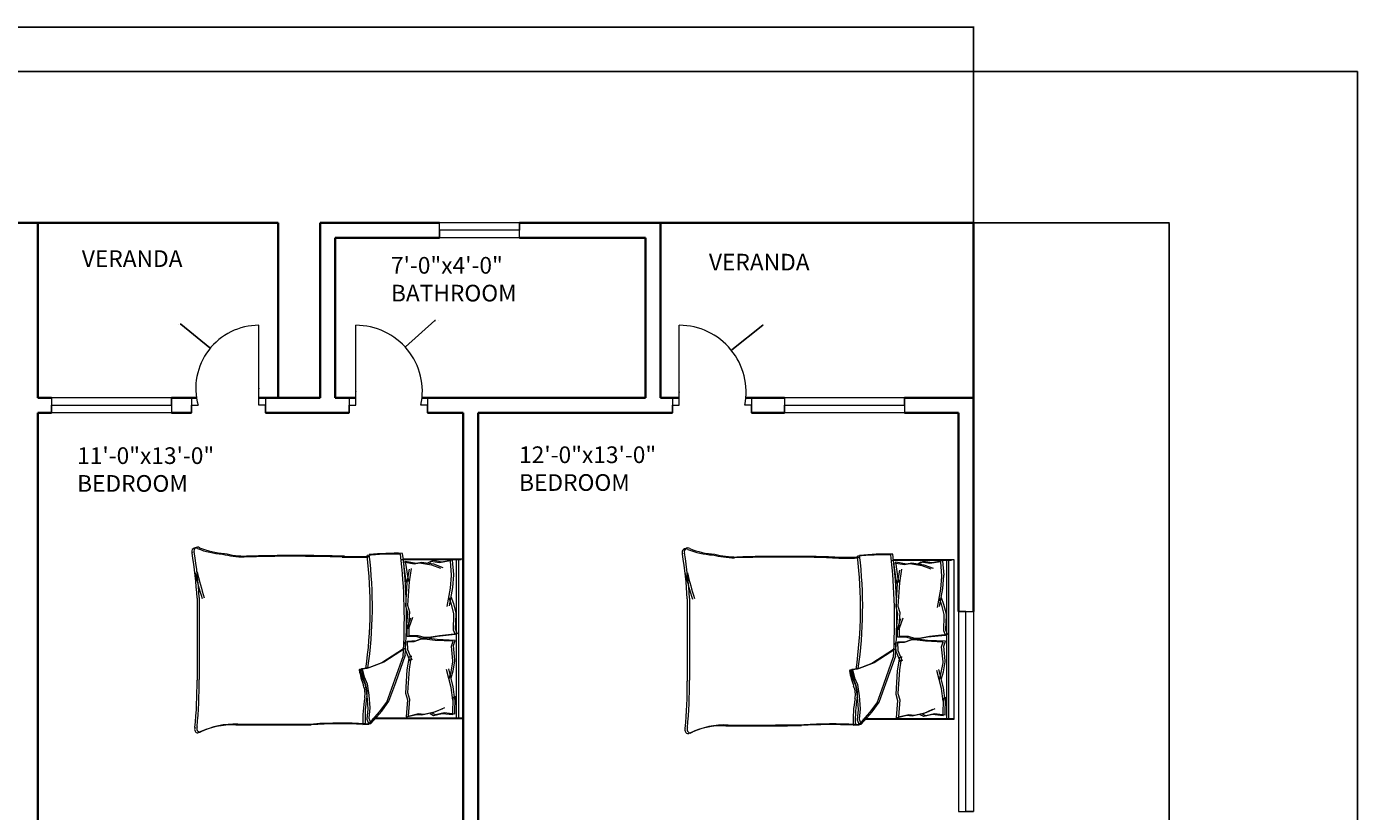
# Model space of a CAD drawing. Units: inches. Extents: x 2163 to 2982, y 1024 to 2288.
# Tile 22 of 22: x 2583 to 2982, y 2053 to 2288. Entities that reach past the tile are written whole.
import ezdxf

# ---------------------------------------------------------------- set-up
doc = ezdxf.new("R2010")
doc.units = ezdxf.units.IN
for name, color, linetype, lineweight in [('A-ANNO-DIMS', 2, 'Continuous', 18), ('A-ANNO-TTLB', 7, 'Continuous', 25), ('A-AREA-IDEN', 7, 'Continuous', 18), ('A-DOOR', 11, 'Continuous', 18), ('A-FURN', 8, 'Continuous', 13), ('A-GLAZ', 161, 'Continuous', 18), ('A-WALL', 7, 'Continuous', 35)]:
    doc.layers.add(name, color=color, linetype=linetype, lineweight=lineweight)
doc.styles.get("Standard").update_dxf_attribs({"font": 'arial.ttf'})
doc.dimstyles.get("Standard").update_dxf_attribs({"dimtxt": 0.18, "dimasz": 0.18, "dimexe": 0.18, "dimexo": 0.0625, "dimgap": 0.09, "dimtad": 0, "dimtih": 1, "dimtoh": 1, "dimdec": 4, "dimzin": 0, "dimdsep": 46, "dimtxsty": 'Standard', "dimcen": 0.09, "dimadec": 0, "dimazin": 0, "dimtfac": 1, "dimtdec": 4, "dimtofl": 0, "dimtmove": 0, "dimatfit": 3, "dimfxl": 1, "dimtolj": 1, "dimtzin": 0, "dimarcsym": 0})

# ---------------------------------------------------------------- blocks, each defined once
blk = doc.blocks.new('BED-DOUBLE')
for p, q in [((27.75, 52.87), (24.5, 49.16)), ((27.75, 52.87), (24.5, 49.16)), ((28.38, 53.1), (25.13, 49.39)), ((28.38, 53.1), (25.13, 49.39)), ((29.49, 52.95), (27.75, 52.87, 3.87)), ((29.49, 52.95), (27.75, 52.87, 3.87)), ((28.36, 51.33), (27.75, 52.87)), ((28.36, 51.33), (27.75, 52.87)), ((30.13, 53.18), (28.38, 53.1, 3.87)), ((29, 51.56), (28.38, 53.1)), ((30.13, 53.18), (28.38, 53.1, 3.87)), ((29, 51.56), (28.38, 53.1)), ((0, 51.49), (0.64, 51.49)), ((0, 3.47), (0, 51.49)), ((0, 51.27), (26.61, 51.27)), ((0, 51.27), (26.61, 51.27)), ((0.64, 51.49), (27.25, 51.49)), ((0.64, 51.49), (27.25, 51.49)), ((1.53, 3.48), (1.53, 51.27)), ((1.53, 3.47), (1.53, 51.27)), ((2.17, 3.7), (2.17, 51.49)), ((2.17, 3.7), (2.17, 51.49)), ((2.56, 50.11), (2.46, 44.71)), ((2.56, 50.11), (2.46, 44.71)), ((2.56, 50.11), (5.77, 49.73)), ((2.56, 50.11), (5.77, 49.73)), ((3.2, 50.34), (3.1, 44.94)), ((3.2, 50.34), (3.1, 44.94)), ((3.2, 50.34), (6.41, 49.96)), ((3.2, 50.34), (6.41, 49.96)), ((8.26, 49.31), (5.58, 48.13)), ((8.26, 49.31), (5.58, 48.13)), ((5.77, 49.73), (8.34, 50.33)), ((5.77, 49.73), (8.34, 50.33)), ((8.9, 49.54), (6.22, 48.36)), ((8.9, 49.54), (6.22, 48.36)), ((6.41, 49.96), (8.98, 50.56)), ((6.41, 49.96), (8.98, 50.56)), ((11.83, 50.11), (8.26, 49.31)), ((11.83, 50.11), (8.26, 49.31)), ((8.34, 50.33), (9.38, 49.81)), ((8.34, 50.33), (9.38, 49.81)), ((12.47, 50.34), (8.9, 49.54)), ((12.47, 50.34), (8.9, 49.54)), ((8.98, 50.56), (10.02, 50.04)), ((8.98, 50.56), (10.02, 50.04)), ((13.43, 49.92), (11.83, 50.11)), ((13.43, 49.92), (11.83, 50.11)), ((14.07, 50.15), (12.47, 50.34)), ((14.07, 50.15), (12.47, 50.34)), ((16.57, 50.7), (13.43, 49.92)), ((16.57, 50.7), (13.43, 49.92)), ((17.21, 50.93), (14.07, 50.15)), ((17.21, 50.93), (14.07, 50.15)), ((16.17, 45.57), (16.57, 50.7)), ((16.17, 45.57), (16.57, 50.7)), ((16.81, 45.79), (17.21, 50.93)), ((16.81, 45.79), (17.21, 50.93)), ((24.5, 49.16), (22.33, 46.22)), ((24.5, 49.16), (22.33, 46.22)), ((25.13, 49.39), (22.97, 46.45)), ((25.13, 49.39), (22.97, 46.45)), ((28.06, 48.23), (28.36, 51.33)), ((28.06, 48.23), (28.36, 51.33)), ((28.36, 44.36), (28.06, 48.23)), ((28.36, 44.36), (28.06, 48.23)), ((28.69, 48.46), (29, 51.56)), ((28.69, 48.46), (29, 51.56)), ((29, 44.59), (28.69, 48.46)), ((29, 44.59), (28.69, 48.46)), ((2.46, 44.71), (2.54, 45.71)), ((2.46, 44.71), (2.54, 45.71)), ((2.54, 45.71), (3.07, 41.91)), ((2.54, 45.71), (3.07, 41.91)), ((3.1, 44.94), (3.18, 45.94)), ((3.1, 44.94), (3.18, 45.94)), ((3.18, 45.94), (3.71, 42.14)), ((3.18, 45.94), (3.71, 42.14)), ((16.73, 43.61), (16.17, 45.57)), ((16.73, 43.61), (16.17, 45.57)), ((17.37, 43.83), (16.81, 45.79)), ((17.37, 43.83), (16.81, 45.79)), ((22.33, 46.22), (20.32, 40.64)), ((22.33, 46.22), (20.32, 40.64)), ((22.97, 46.45), (20.96, 40.87)), ((22.97, 46.45), (20.96, 40.87)), ((28.83, 40.95), (28.36, 44.36)), ((28.83, 40.95), (28.36, 44.36)), ((29.47, 41.18), (29, 44.59)), ((29.47, 41.18), (29, 44.59)), ((3.07, 41.91), (4.42, 36.49)), ((3.07, 41.91), (4.42, 36.49)), ((3.71, 42.14), (5.06, 36.72)), ((3.71, 42.14), (5.06, 36.72)), ((16.29, 36.6), (16.73, 43.61)), ((16.29, 36.6), (16.73, 43.61)), ((16.93, 36.82), (17.37, 43.83)), ((16.93, 36.82), (17.37, 43.83)), ((20.32, 40.64), (17.38, 32.31)), ((20.32, 40.64), (17.38, 32.31)), ((20.96, 40.87), (18.02, 32.53)), ((20.96, 40.87), (18.02, 32.53)), ((29.76, 38.94), (28.83, 40.95)), ((29.76, 38.94), (28.83, 40.95)), ((30.4, 39.17), (29.47, 41.18)), ((30.4, 39.17), (29.47, 41.18)), ((79.88, 15.29), (79.88, 39.91)), ((79.88, 15.29), (79.88, 39.91)), ((3.08, 37.14), (2.54, 34.2)), ((3.08, 37.13), (2.54, 34.2)), ((3.67, 39.2), (3.08, 37.14)), ((3.67, 39.2), (3.08, 37.13)), ((3.72, 37.36), (3.18, 34.43)), ((3.72, 37.36), (3.18, 34.43)), ((4.31, 39.43), (3.72, 37.36)), ((4.31, 39.43), (3.72, 37.36)), ((15.63, 32.56), (16.29, 36.6)), ((15.63, 32.56), (16.29, 36.6)), ((16.27, 32.79), (16.93, 36.82)), ((16.27, 32.79), (16.93, 36.82)), ((23.88, 34.45), (28.36, 36.15)), ((23.88, 34.45), (28.36, 36.15)), ((24.52, 34.68), (29, 36.38)), ((24.52, 34.68), (29, 36.38)), ((28.36, 36.15), (30.38, 36.46)), ((28.36, 36.15), (30.38, 36.46)), ((29, 36.38), (31.02, 36.69)), ((29, 36.38), (31.02, 36.69)), ((30.38, 36.46), (29.76, 38.94)), ((30.38, 36.46), (29.76, 38.94)), ((31.02, 36.69), (30.4, 39.17)), ((31.02, 36.69), (30.4, 39.17)), ((79.24, 15.06), (79.24, 39.68)), ((79.24, 15.06), (79.24, 39.68)), ((2.54, 34.2), (2.56, 33.88)), ((2.54, 34.2), (2.56, 33.88)), ((2.56, 33.88), (2.98, 29.46)), ((2.56, 33.88), (2.98, 29.46)), ((3.18, 34.43), (3.2, 34.11)), ((3.18, 34.43), (3.2, 34.11)), ((3.2, 34.11), (3.62, 29.68)), ((3.2, 34.11), (3.62, 29.68)), ((16.74, 30.75), (15.45, 33.82)), ((16.74, 30.75), (15.45, 33.82)), ((17.38, 30.98), (16.09, 34.05)), ((17.38, 30.98), (16.09, 34.05)), ((17.38, 30.26), (23.88, 34.45)), ((17.38, 30.26), (23.88, 34.45)), ((18.02, 30.49), (24.52, 34.68)), ((18.02, 30.49), (24.52, 34.68)), ((2.98, 29.46), (2.49, 27.98)), ((2.98, 29.46), (2.49, 27.98)), ((2.49, 27.98), (7.87, 27.73)), ((2.49, 27.98), (7.87, 27.73)), ((3.62, 29.68), (3.13, 28.21)), ((3.62, 29.68), (3.13, 28.2)), ((3.13, 28.21), (8.51, 27.96)), ((3.13, 28.2), (8.51, 27.96)), ((8.51, 27.96), (11.72, 27.58)), ((8.51, 27.96), (11.72, 27.58)), ((12.38, 27.44), (14.22, 28.13)), ((12.38, 27.44), (14.22, 28.13)), ((13.02, 27.66), (14.86, 28.36)), ((13.02, 27.66), (14.86, 28.36)), ((14.22, 28.13), (16.89, 28.3)), ((14.22, 28.13), (16.89, 28.3)), ((14.86, 28.36), (17.53, 28.53)), ((14.86, 28.36), (17.53, 28.53)), ((16.89, 28.3), (16.74, 30.75)), ((16.89, 28.3), (16.74, 30.75)), ((17.53, 28.53), (17.38, 30.98)), ((17.53, 28.53), (17.38, 30.98)), ((1.87, 25.98), (7.22, 26.56)), ((1.87, 25.98), (7.22, 26.56)), ((2.45, 24.54), (1.87, 25.98)), ((2.45, 24.54), (1.87, 25.98)), ((2.3, 20.09), (2.45, 24.54)), ((2.3, 20.09), (2.45, 24.54)), ((2.51, 26.21), (7.86, 26.79)), ((2.51, 26.21), (7.86, 26.79)), ((3.09, 24.77), (2.51, 26.21)), ((3.09, 24.77), (2.51, 26.21)), ((2.94, 20.32), (3.09, 24.77)), ((2.94, 20.32), (3.09, 24.77)), ((7.22, 26.56), (10.4, 27.14)), ((7.22, 26.56), (10.4, 27.14)), ((7.86, 26.79), (11.04, 27.37)), ((7.86, 26.79), (11.04, 27.37)), ((7.87, 27.73), (11.08, 27.35)), ((7.87, 27.73), (11.08, 27.35)), ((10.4, 27.14), (11.7, 27.14)), ((10.4, 27.14), (11.7, 27.14)), ((11.04, 27.37), (12.34, 27.37)), ((11.04, 27.37), (12.34, 27.37)), ((11.08, 27.35), (12.38, 27.44)), ((11.08, 27.35), (12.38, 27.44)), ((11.7, 27.14), (13.58, 26.56)), ((11.7, 27.14), (13.58, 26.56)), ((11.72, 27.58), (13.02, 27.66)), ((11.72, 27.58), (13.02, 27.66)), ((12.34, 27.37), (14.22, 26.79)), ((12.34, 27.37), (14.22, 26.79)), ((13.58, 26.56), (16.26, 26.56)), ((13.58, 26.56), (16.26, 26.56)), ((14.22, 26.79), (16.9, 26.79)), ((14.22, 26.79), (16.9, 26.79)), ((16.26, 24.1), (15.17, 20.96)), ((16.26, 24.1), (15.17, 20.96)), ((16.9, 24.33), (15.81, 21.19)), ((16.9, 24.33), (15.81, 21.19)), ((16.17, 19.38), (16.57, 24.52)), ((16.17, 19.38), (16.57, 24.52)), ((16.26, 26.56), (16.26, 24.1)), ((16.26, 26.56), (16.26, 24.1)), ((16.81, 19.61), (17.21, 24.74)), ((16.81, 19.61), (17.21, 24.74)), ((16.9, 26.79), (16.9, 24.33)), ((16.9, 26.79), (16.9, 24.33)), ((2.3, 19.77), (2.3, 20.09)), ((2.3, 19.77), (2.3, 20.09)), ((2.94, 20), (2.94, 20.32)), ((2.94, 20), (2.94, 20.32)), ((3.67, 17.11), (2.94, 20)), ((3.67, 17.11), (2.94, 20)), ((3.03, 16.88), (2.3, 19.77)), ((3.03, 16.88), (2.3, 19.77)), ((3.75, 14.85), (3.03, 16.88)), ((3.75, 14.85), (3.03, 16.88)), ((3.32, 12.11), (4.33, 17.6)), ((3.32, 12.11), (4.33, 17.6)), ((4.39, 15.08), (3.67, 17.11)), ((4.39, 15.08), (3.67, 17.11)), ((3.96, 12.34), (4.97, 17.83)), ((3.96, 12.34), (4.97, 17.83)), ((16.73, 17.42), (16.17, 19.38)), ((16.73, 17.42), (16.17, 19.38)), ((16.29, 10.41), (16.73, 17.42)), ((16.29, 10.41), (16.73, 17.42)), ((17.37, 17.65), (16.81, 19.61)), ((17.37, 17.65), (16.81, 19.61)), ((16.93, 10.64), (17.37, 17.65)), ((16.93, 10.64), (17.37, 17.65)), ((3.03, 8.28), (3.32, 12.11)), ((3.03, 8.28), (3.32, 12.11)), ((3.67, 8.51), (3.96, 12.34)), ((3.67, 8.51), (3.96, 12.34)), ((3.01, 8.18), (3.03, 8.28)), ((3.01, 8.18), (3.03, 8.28)), ((3.34, 3.9), (3.01, 8.18)), ((3.34, 3.9), (3.01, 8.18)), ((3.65, 8.41), (3.67, 8.51)), ((3.65, 8.41), (3.67, 8.51)), ((3.98, 4.13), (3.65, 8.41)), ((3.98, 4.13), (3.65, 8.41)), ((15.63, 6.38), (16.29, 10.41)), ((15.63, 6.38), (16.29, 10.41)), ((16.27, 6.61), (16.93, 10.64)), ((16.27, 6.61), (16.93, 10.64)), ((16.29, 10.41), (16.62, 9.28)), ((16.29, 10.41), (16.62, 9.28)), ((16.62, 9.28), (17.34, 4.18)), ((16.62, 9.28), (17.34, 4.18)), ((16.93, 10.64), (17.26, 9.51)), ((16.93, 10.64), (17.26, 9.51)), ((17.26, 9.51), (17.98, 4.41)), ((17.26, 9.51), (17.98, 4.41)), ((3.32, 3.89), (6.5, 4.47)), ((3.32, 3.89), (6.5, 4.47)), ((3.96, 4.12), (7.14, 4.7)), ((3.96, 4.12), (7.14, 4.7)), ((8.95, 5.05), (6.21, 6.06)), ((8.95, 5.05), (6.21, 6.06)), ((6.5, 4.47), (9.1, 4.04)), ((6.5, 4.47), (9.1, 4.04)), ((9.59, 5.28), (6.85, 6.29)), ((9.59, 5.28), (6.85, 6.29)), ((7.14, 4.7), (9.74, 4.27)), ((7.14, 4.7), (9.74, 4.27)), ((12.57, 4.47), (8.95, 5.05)), ((12.57, 4.47), (8.95, 5.05)), ((9.1, 4.04), (10.11, 4.62)), ((9.1, 4.04), (10.11, 4.62)), ((13.21, 4.7), (9.59, 5.28)), ((13.21, 4.7), (9.59, 5.28)), ((9.74, 4.27), (10.75, 4.85)), ((9.74, 4.27), (10.75, 4.85)), ((14.16, 4.76), (12.57, 4.47)), ((14.16, 4.76), (12.57, 4.47)), ((14.8, 4.99), (13.21, 4.7)), ((14.8, 4.99), (13.21, 4.7)), ((17.34, 4.18), (14.16, 4.76)), ((17.34, 4.18), (14.16, 4.76)), ((17.98, 4.41), (14.8, 4.99)), ((17.98, 4.41), (14.8, 4.99)), ((18.11, 3.48), (0, 3.48)), ((18.11, 3.47), (0, 3.47)), ((18.75, 3.7), (0.64, 3.7)), ((18.75, 3.7), (0.64, 3.7))]:
    blk.add_line(p, q)
for centre, radius, start, end in [((-6.66, 51.33), 36.18, 349.8763, 2.5657), ((-6.66, 51.33), 36.18, 349.8763, 2.5657), ((36.31, 182.27), 129.5, 266.9791, 273.8365), ((36.31, 182.27), 129.5, 266.9791, 273.8365), ((-6.02, 51.56), 36.18, 349.8763, 2.5657), ((-6.02, 51.56), 36.18, 349.8763, 2.5657), ((36.95, 182.49), 129.5, 266.9791, 273.8365), ((36.95, 182.49), 129.5, 266.9791, 273.8365), ((67.82, -4508.74), 4561.86, 90.00217, 90.28689), ((67.82, -4508.74), 4561.86, 90.00217, 90.28689), ((68.46, -4508.52), 4561.86, 90.00217, 90.28689), ((68.46, -4508.52), 4561.86, 90.00217, 90.28689), ((68.67, 76.16), 23.07, 267.4714, 296.4681), ((68.67, 76.16), 23.07, 267.4714, 296.4681), ((69.31, 76.39), 23.07, 267.4714, 296.4681), ((69.31, 76.39), 23.07, 267.4714, 296.4681), ((78.87, 54.41), 1.1, 332.6588, 86.02), ((78.87, 54.41), 1.1, 332.6588, 86.02), ((212.28, 41.15), 133.04, 174.4998, 180.6351), ((212.28, 41.15), 133.04, 174.4998, 180.6351), ((79.51, 54.64), 1.1, 332.6588, 86.02), ((79.51, 54.64), 1.1, 332.6588, 86.02), ((212.92, 41.38), 133.04, 174.4998, 180.6351), ((212.92, 41.38), 133.04, 174.4998, 180.6351), ((35.07, 43.74), 6.22, 168.6608, 203.7384), ((35.07, 43.74), 6.22, 168.6608, 203.7384), ((35.71, 43.97), 6.22, 168.6608, 203.7384), ((35.71, 43.97), 6.22, 168.6608, 203.7384), ((1.48, 31.15), 29.65, 10.6617, 19.8806), ((1.48, 31.15), 29.65, 10.6617, 19.8806), ((2.12, 31.38), 29.65, 10.6617, 19.8806), ((2.12, 31.38), 29.65, 10.6617, 19.8806), ((156.32, 17.76), 129.02, 171.7845, 186.9006), ((156.32, 17.76), 129.02, 171.7845, 186.9006), ((156.96, 17.98), 129.02, 171.7845, 186.9006), ((156.96, 17.98), 129.02, 171.7845, 186.9006), ((30.44, 36.64), 0.185, 250.2464, 1.1377), ((30.44, 36.64), 0.185, 250.2464, 1.1377), ((31.08, 36.86), 0.185, 250.2464, 1.1377), ((31.08, 36.86), 0.185, 250.2464, 1.1377), ((182.05, 21.36), 164.97, 176.0865, 186.7821), ((182.05, 21.36), 164.97, 176.0865, 186.7821), ((182.69, 21.59), 164.97, 176.0865, 186.7821), ((182.69, 21.59), 164.97, 176.0865, 186.7821), ((-23.71, -17.22), 106.46, 13.3832, 17.7053), ((-23.71, -17.22), 106.46, 13.3832, 17.7053), ((-23.07, -16.99), 106.46, 13.3832, 17.7053), ((-23.07, -16.99), 106.46, 13.3832, 17.7053), ((200.84, 21.43), 121.76, 182.9958, 189.4091), ((200.84, 21.43), 121.76, 182.9958, 189.4091), ((201.48, 21.66), 121.76, 182.9958, 189.4091), ((201.48, 21.65), 121.76, 182.9958, 189.4091), ((20.1, 85.16), 83.31, 268.7218, 275.604), ((20.1, 85.16), 83.31, 268.7218, 275.604), ((20.74, 85.39), 83.31, 268.7218, 275.604), ((20.74, 85.39), 83.31, 268.7218, 275.604), ((31.17, -167.31), 170.11, 88.4762, 91.0082), ((31.17, -167.31), 170.11, 88.4762, 91.0082), ((31.81, -167.08), 170.11, 88.4762, 91.0082), ((31.81, -167.08), 170.11, 88.4762, 91.0082), ((50.61, 484.82), 482.31, 268.2277, 271.7185), ((50.61, 484.82), 482.31, 268.2277, 271.7185), ((51.25, 485.05), 482.31, 268.2277, 271.7185), ((51.25, 485.05), 482.31, 268.2277, 271.7185), ((64.51, -26.9), 29.63, 76.0648, 88.9113), ((64.51, -26.9), 29.63, 76.0648, 88.9113), ((65.15, -26.67), 29.63, 76.0648, 88.9113), ((65.15, -26.67), 29.63, 76.0648, 88.9113), ((70.28, -21.66), 23.56, 67.9751, 86.652), ((70.28, -21.66), 23.56, 67.9751, 86.652), ((70.91, -21.43), 23.56, 67.9751, 86.652), ((70.91, -21.43), 23.56, 67.9751, 86.652), ((79.72, 1.09), 1.09, 236.1736, 23.4781), ((79.72, 1.09), 1.09, 236.1736, 23.4781), ((80.36, 1.32), 1.09, 236.1736, 23.4781), ((80.36, 1.32), 1.09, 236.1736, 23.4781)]:
    blk.add_arc(centre, radius, start, end)
blk = doc.blocks.new('WIN-24')
for p, q in [((0, 24), (4.5, 24)), ((0, 24), (0, 0)), ((4.5, 24), (2.25, 24)), ((2.25, 24), (2.25, 0)), ((4.5, 24), (4.5, 0)), ((2.25, 0), (0, 0)), ((0, 0), (4.5, 0))]:
    blk.add_line(p, q)
blk = doc.blocks.new('WIN-60')
for p, q in [((2.25, 60), (0, 60)), ((0, 60), (4.5, 60)), ((0, 60), (0, 0)), ((2.25, 0), (2.25, 60)), ((4.5, 60), (4.5, 0)), ((0, 0), (4.5, 0)), ((4.5, 0), (2.25, 0))]:
    blk.add_line(p, q)
blk = doc.blocks.new('WIN-36')
for p, q in [((2.25, 36), (0, 36)), ((0, 36), (4.5, 36)), ((0, 36), (0, 0)), ((2.25, 0), (2.25, 36)), ((4.5, 36), (4.5, 0)), ((0, 0), (4.5, 0)), ((4.5, 0), (2.25, 0))]:
    blk.add_line(p, q)
blk = doc.blocks.new('*D29')
at = {"layer": 'A-ANNO-DIMS', "color": 0, "lineweight": -2, "transparency": 16777216}
for p, q in [((2285.34, 1738.83), (2285.34, 2288.1)), ((2285.52, 2287.92), (2576.05, 2287.92)), ((2867.16, 2287.92), (2576.63, 2287.92)), ((2867.34, 2229.33), (2867.34, 2288.1))]:
    blk.add_line(p, q, dxfattribs=at)
at = {"layer": 'A-ANNO-DIMS', "color": 0, "transparency": 16777216}
for points in [[(2285.52, 2287.95), (2285.52, 2287.89), (2285.34, 2287.92)], [(2867.16, 2287.95), (2867.16, 2287.89), (2867.34, 2287.92)]]:
    blk.add_solid(points, dxfattribs=at)
at = {"layer": 'Defpoints', "color": 0, "transparency": 16777216}
for p in [(2867.34, 2287.92), (2867.34, 2229.27), (2285.34, 1738.77)]:
    blk.add_point(p, dxfattribs=at)
at = {"layer": 'A-ANNO-DIMS', "color": 0, "transparency": 16777216, "insert": (2576.34, 2287.92), "char_height": 0.18, "attachment_point": 5}
blk.add_mtext('\\A1;582', dxfattribs=at)
blk = doc.blocks.new('*D31')
at = {"layer": 'A-ANNO-DIMS', "color": 0, "lineweight": -2, "transparency": 16777216}
for p, q in [((2867.4, 2229.27), (2926.17, 2229.27)), ((2925.99, 2229.09), (2925.99, 1957.95)), ((2925.99, 1686.45), (2925.99, 1957.59)), ((2862.9, 1686.27), (2926.17, 1686.27))]:
    blk.add_line(p, q, dxfattribs=at)
at = {"layer": 'A-ANNO-DIMS', "color": 0, "transparency": 16777216}
for points in [[(2925.96, 2229.09), (2926.02, 2229.09), (2925.99, 2229.27)], [(2925.96, 1686.45), (2926.02, 1686.45), (2925.99, 1686.27)]]:
    blk.add_solid(points, dxfattribs=at)
at = {"layer": 'Defpoints', "color": 0, "transparency": 16777216}
for p in [(2867.34, 2229.27), (2925.99, 2229.27), (2862.84, 1686.27)]:
    blk.add_point(p, dxfattribs=at)
at = {"layer": 'A-ANNO-DIMS', "color": 0, "transparency": 16777216, "insert": (2925.99, 1957.77), "char_height": 0.18, "attachment_point": 5}
blk.add_mtext('\\A1;543', dxfattribs=at)
blk = doc.blocks.new('*D32')
at = {"layer": 'A-ANNO-DIMS', "color": 0, "lineweight": -2, "transparency": 16777216}
for p, q in [((2867.4, 2229.27), (2926.17, 2229.27)), ((2925.99, 2229.09), (2925.99, 1686.35)), ((2925.99, 1143.25), (2925.99, 1685.99)), ((2867.4, 1143.07), (2926.17, 1143.07))]:
    blk.add_line(p, q, dxfattribs=at)
at = {"layer": 'A-ANNO-DIMS', "color": 0, "transparency": 16777216}
for points in [[(2925.96, 2229.09), (2926.02, 2229.09), (2925.99, 2229.27)], [(2925.96, 1143.25), (2926.02, 1143.25), (2925.99, 1143.07)]]:
    blk.add_solid(points, dxfattribs=at)
at = {"layer": 'Defpoints', "color": 0, "transparency": 16777216}
for p in [(2867.34, 2229.27), (2925.99, 2229.27), (2867.34, 1143.07)]:
    blk.add_point(p, dxfattribs=at)
at = {"layer": 'A-ANNO-DIMS', "color": 0, "transparency": 16777216, "insert": (2925.99, 1686.17), "char_height": 0.18, "attachment_point": 5}
blk.add_mtext('\\A1;1086.2', dxfattribs=at)
blk = doc.blocks.new('*D60')
at = {"layer": 'A-ANNO-DIMS', "color": 0, "lineweight": -2, "transparency": 16777216}
for p, q in [((2629.52, 2198.81), (2629.7, 2198.81)), ((2629.7, 2198.81), (2638.35, 2191.71)), ((2653.04, 2179.57), (2653.22, 2179.57)), ((2653.13, 2179.48), (2653.13, 2179.66))]:
    blk.add_line(p, q, dxfattribs=at)
at = {"layer": 'A-ANNO-DIMS', "color": 0, "transparency": 16777216}
blk.add_solid([(2638.37, 2191.74), (2638.33, 2191.69), (2638.49, 2191.6)], dxfattribs=at)
at = {"layer": 'Defpoints', "color": 0, "transparency": 16777216}
for p in [(2638.49, 2191.6), (2653.13, 2179.57)]:
    blk.add_point(p, dxfattribs=at)
at = {"layer": 'A-ANNO-DIMS', "color": 0, "transparency": 16777216, "insert": (2628.98, 2198.81), "char_height": 0.18, "attachment_point": 5}
blk.add_mtext('\\A1;R18.944', dxfattribs=at)
blk = doc.blocks.new('*D61')
at = {"layer": 'A-ANNO-DIMS', "color": 0, "lineweight": -2, "transparency": 16777216}
for p, q in [((2705.83, 2199.99), (2697.09, 2192.09)), ((2706.01, 2199.99), (2705.83, 2199.99)), ((2682.1, 2178.59), (2682.28, 2178.59)), ((2682.19, 2178.5), (2682.19, 2178.68))]:
    blk.add_line(p, q, dxfattribs=at)
at = {"layer": 'A-ANNO-DIMS', "color": 0, "transparency": 16777216}
blk.add_solid([(2697.07, 2192.11), (2697.11, 2192.06), (2696.96, 2191.96)], dxfattribs=at)
at = {"layer": 'Defpoints', "color": 0, "transparency": 16777216}
for p in [(2696.96, 2191.96), (2682.19, 2178.59)]:
    blk.add_point(p, dxfattribs=at)
at = {"layer": 'A-ANNO-DIMS', "color": 0, "transparency": 16777216, "insert": (2706.49, 2199.99), "char_height": 0.18, "attachment_point": 5}
blk.add_mtext('\\A1;R19.93', dxfattribs=at)
blk = doc.blocks.new('*D62')
at = {"layer": 'A-ANNO-DIMS', "color": 0, "lineweight": -2, "transparency": 16777216}
for p, q in [((2804.16, 2198.55), (2794.92, 2191.13)), ((2804.34, 2198.55), (2804.16, 2198.55)), ((2779.06, 2178.47), (2779.24, 2178.47)), ((2779.15, 2178.38), (2779.15, 2178.56))]:
    blk.add_line(p, q, dxfattribs=at)
at = {"layer": 'A-ANNO-DIMS', "color": 0, "transparency": 16777216}
blk.add_solid([(2794.9, 2191.16), (2794.94, 2191.11), (2794.78, 2191.02)], dxfattribs=at)
at = {"layer": 'Defpoints', "color": 0, "transparency": 16777216}
for p in [(2794.78, 2191.02), (2779.15, 2178.47)]:
    blk.add_point(p, dxfattribs=at)
at = {"layer": 'A-ANNO-DIMS', "color": 0, "transparency": 16777216, "insert": (2804.82, 2198.55), "char_height": 0.18, "attachment_point": 5}
blk.add_mtext('\\A1;R20.05', dxfattribs=at)

msp = doc.modelspace()

# ---------------------------------------------------------------- linework, layer by layer
at = {"layer": 'A-ANNO-TTLB'}
msp.add_lwpolyline([(2162.6841, 2274.6054), (2982.469, 2274.6054), (2982.469, 1045.9691), (2162.6841, 1045.9691)], close=True, dxfattribs=at)
at = {"layer": 'A-DOOR'}
for p, q in [((2653.1269, 2174.5188), (2653.1269, 2198.5188)), ((2682.1865, 2174.5188), (2682.1865, 2198.5188)), ((2779.1453, 2174.5188), (2779.1453, 2198.5188)), ((2632.8695, 2176.7688), (2632.8695, 2172.2688)), ((2655.1269, 2176.7688), (2655.1269, 2172.2688)), ((2680.1865, 2176.7688), (2680.1865, 2172.2688)), ((2703.697, 2176.7688), (2703.697, 2172.2688)), ((2777.1453, 2176.7688), (2777.1453, 2172.2688)), ((2800.8036, 2176.7688), (2800.8036, 2172.2688)), ((2632.8695, 2172.2688), (2632.8695, 2174.5188)), ((2632.8695, 2174.5188), (2634.8695, 2174.5188)), ((2655.1269, 2174.5188), (2653.1269, 2174.5188)), ((2655.1269, 2172.2688), (2655.1269, 2174.5188)), ((2680.1865, 2172.2688), (2680.1865, 2174.5188)), ((2680.1865, 2174.5188), (2682.1865, 2174.5188)), ((2703.697, 2174.5188), (2701.697, 2174.5188)), ((2703.697, 2172.2688), (2703.697, 2174.5188)), ((2777.1453, 2172.2688), (2777.1453, 2174.5188)), ((2777.1453, 2174.5188), (2779.1453, 2174.5188)), ((2800.8036, 2174.5188), (2798.8036, 2174.5188)), ((2800.8036, 2172.2688), (2800.8036, 2174.5188))]:
    msp.add_line(p, q, dxfattribs=at)
for centre, radius, start, end in [((2653.1269, 2179.5744), 18.9444, 90, 195.477728), ((2682.1865, 2178.5885), 19.9304, 348.21777, 90), ((2779.1453, 2178.4679), 20.0509, 348.641269, 90)]:
    msp.add_arc(centre, radius, start, end, dxfattribs=at)
at = {"layer": 'A-WALL'}
for p, q in [((2586.8389, 2229.2688), (2510.3389, 2229.2688)), ((2586.8389, 2176.7688), (2586.8389, 2229.2688)), ((2586.8389, 2229.2688), (2658.8389, 2229.2688)), ((2586.8389, 2229.2688), (2658.8389, 2229.2688)), ((2658.8389, 2229.2688), (2658.8389, 2176.7688)), ((2671.4905, 2176.7688), (2671.4905, 2229.2688)), ((2671.4905, 2229.2688), (2707.2643, 2229.2688)), ((2731.2643, 2229.2688), (2769.0635, 2229.2688)), ((2759.9905, 2229.2688), (2755.4905, 2229.2688)), ((2769.0635, 2229.2688), (2773.5635, 2229.2688)), ((2867.3389, 2229.2688), (2773.5635, 2229.2688)), ((2773.5635, 2229.2688), (2773.5635, 2176.7688)), ((2867.3389, 2176.7688), (2867.3389, 2229.2688)), ((2675.9905, 2224.7688), (2675.9905, 2176.7688)), ((2707.2643, 2224.7688), (2675.9905, 2224.7688)), ((2769.0635, 2224.7688), (2731.2643, 2224.7688)), ((2769.0635, 2176.7688), (2769.0635, 2224.7688)), ((2586.8389, 2176.7688), (2590.9121, 2176.7688)), ((2626.9121, 2176.7688), (2634.3914, 2176.7688)), ((2653.1269, 2176.7688), (2671.4905, 2176.7688)), ((2675.9905, 2176.7688), (2682.1865, 2176.7688)), ((2702.0337, 2176.7688), (2769.0635, 2176.7688)), ((2755.4905, 2176.7688), (2759.9905, 2176.7688)), ((2773.5635, 2176.7688), (2779.1453, 2176.7688)), ((2799.1242, 2176.7688), (2810.6963, 2176.7688)), ((2846.6963, 2176.7688), (2867.3389, 2176.7688)), ((2867.3389, 2176.7688), (2867.3389, 2112.7024)), ((2586.8389, 2172.2688), (2586.8389, 2016.2688)), ((2586.8389, 2172.2688), (2590.9121, 2172.2688)), ((2626.9121, 2172.2688), (2632.8695, 2172.2688)), ((2655.1269, 2172.2688), (2680.1865, 2172.2688)), ((2703.697, 2172.2688), (2714.3389, 2172.2688)), ((2714.3389, 2172.2688), (2714.3389, 2016.2688)), ((2718.8389, 2172.2688), (2718.8389, 2016.2688)), ((2718.8389, 2172.2688), (2777.1453, 2172.2688)), ((2800.8036, 2172.2688), (2810.6963, 2172.2688)), ((2846.6963, 2172.2688), (2862.8389, 2172.2688)), ((2862.8389, 2172.2688), (2862.8389, 2112.7024))]:
    msp.add_line(p, q, dxfattribs=at)

# ---------------------------------------------------------------- block references
at = {"layer": 'A-FURN', "rotation": 180}
for p in [(2714.4401, 2131.9626), (2861.44, 2131.7171)]:
    msp.add_blockref('BED-DOUBLE', p, dxfattribs=at)
at = {"layer": 'A-GLAZ', "extrusion": (0, 0, -1), "zscale": -1, "rotation": 90}
msp.add_blockref('WIN-24', (-2707.2647, 2224.7689), dxfattribs=at)
at = {"layer": 'A-GLAZ', "rotation": 270}
for p in [(2590.9117, 2176.7688), (2810.6958, 2176.7688)]:
    msp.add_blockref('WIN-36', p, dxfattribs=at)
at = {"layer": 'A-GLAZ'}
msp.add_blockref('WIN-60', (2862.839, 2052.7023), dxfattribs=at)

# ---------------------------------------------------------------- texts
at = {"layer": 'A-AREA-IDEN', "char_height": 5, "attachment_point": 1}
for s, width, insert in [('VERANDA', 43.46851, (2600.0181, 2221.0009)), ('7\'-0"x4\'-0"\\PBATHROOM', 67.322585, (2692.7074, 2218.9967)), ('VERANDA', 44.373288, (2788.0431, 2219.9486)), ('11\'-0"x13\'-0"\\PBEDROOM', 113.250466, (2598.6088, 2161.909)), ('12\'-0"x13\'-0"\\PBEDROOM', 92.770218, (2731.1191, 2162.1825))]:
    msp.add_mtext_dynamic_manual_height_columns(s, width=width, gutter_width=12.5, heights=[0], dxfattribs=dict(at, insert=insert))

# ---------------------------------------------------------------- dimensions: what is measured, and where the dimension line sits
at = {"layer": 'A-ANNO-DIMS'}
dim = msp.add_linear_dim(base=(2867.3389, 2287.9188), p1=(2285.3389, 1738.7688), p2=(2867.3389, 2229.2688), dimstyle='Standard', override={"dimdec": 0, "dimlfac": 1, "dimrnd": 0, "dimzin": 0, "dimdsep": 46, "dimlunit": 2}, dxfattribs=at)
dim.commit()
dim.dimension.update_dxf_attribs({"geometry": '*D29', "text_midpoint": (2576.3389, 2287.9188)})
for p1, override, picture, middle in [((2862.8389, 1686.2688), {"dimdec": 0, "dimlfac": 1, "dimrnd": 0, "dimzin": 0, "dimdsep": 46, "dimlunit": 2}, '*D31', (2925.9889, 1957.7688)), ((2867.3389, 1143.0732), {"dimdec": 1, "dimlfac": 1, "dimrnd": 0, "dimzin": 0, "dimdsep": 46, "dimlunit": 2}, '*D32', (2925.9889, 1686.171))]:
    dim = msp.add_linear_dim(base=(2925.9889, 2229.2688), p1=p1, p2=(2867.3389, 2229.2688), angle=90, dimstyle='Standard', override=override, dxfattribs=at)
    dim.commit()
    dim.dimension.update_dxf_attribs({"geometry": picture, "text_midpoint": middle})
for center, mpoint, override, picture, middle in [((2653.1269, 2179.5744), (2638.488, 2191.5991), {"dimdec": 3, "dimlfac": 1, "dimrnd": 0, "dimzin": 0, "dimdsep": 46, "dimlunit": 2}, '*D60', (2628.9753, 2198.8139)), ((2682.1865, 2178.5885), (2696.9612, 2191.9649), {"dimdec": 2, "dimlfac": 1, "dimrnd": 0, "dimzin": 0, "dimdsep": 46, "dimlunit": 2}, '*D61', (2706.4859, 2199.9907)), ((2779.1453, 2178.4679), (2794.7806, 2191.021), {"dimdec": 2, "dimlfac": 1, "dimrnd": 0, "dimzin": 0, "dimdsep": 46, "dimlunit": 2}, '*D62', (2804.8222, 2198.5528))]:
    dim = msp.add_radius_dim(center=center, mpoint=mpoint, dimstyle='Standard', override=override, dxfattribs=at)
    dim.commit()
    dim.dimension.update_dxf_attribs({"geometry": picture, "text_midpoint": middle, "dimtype": 164})

doc.saveas('drawing.dxf')
